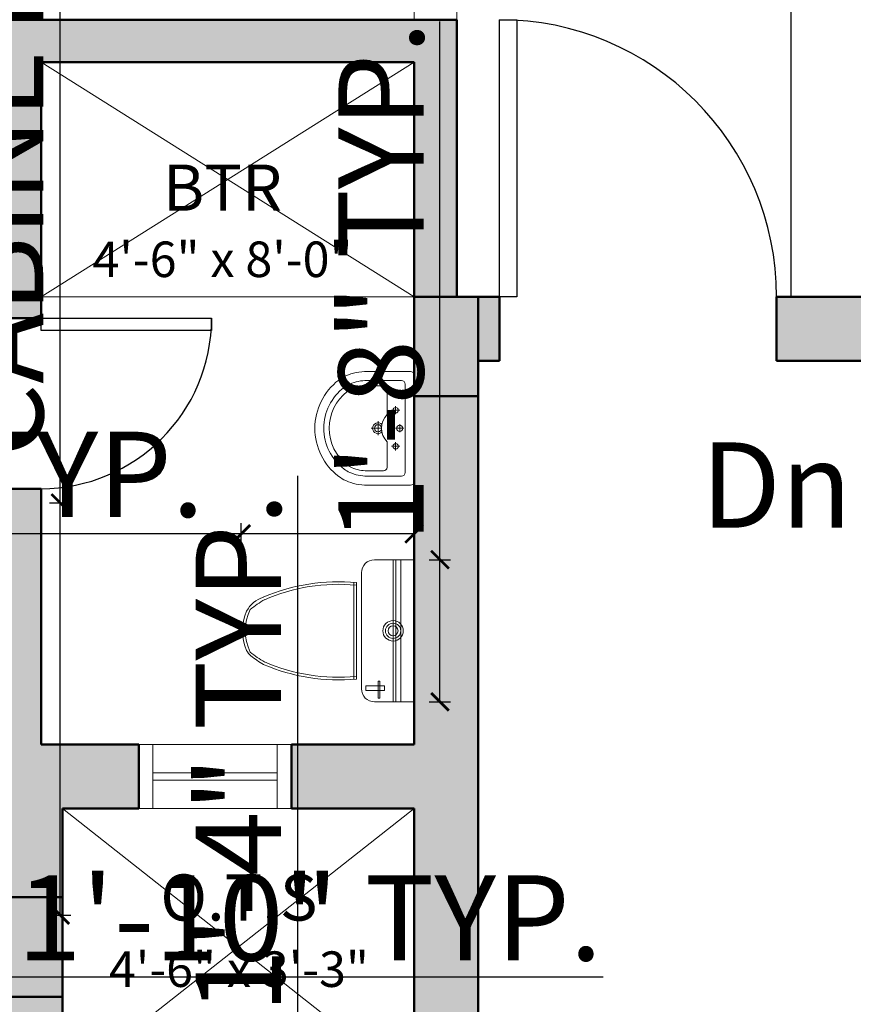
# Model space of a CAD drawing. Units: inches. Extents: x 375 to 1122, y 27 to 1069.
# Tile 80 of 155: x 667 to 784, y 577 to 716. Entities that reach past the tile are written whole.
import ezdxf

# ---------------------------------------------------------------- set-up
doc = ezdxf.new("R2010")
doc.units = ezdxf.units.IN
doc.linetypes.add('ACAD_ISO03W100', pattern=[30, 12, -18])
for name, color, linetype, lineweight in [('A-ANNO-DIMS', 2, 'Continuous', 18), ('A-ANNO-TEXT', 7, 'Continuous', 18), ('A-AREA-IDEN', 7, 'Continuous', 18), ('A-COLS-PATT', 10, 'Continuous', 13), ('A-FLOR-FIXT', 55, 'Continuous', 18), ('A-FLOR-MILL', 55, 'Continuous', 25), ('A-FLOR-OPEN', 250, 'Continuous', 18), ('A-WALL-OVHD', 77, 'ACAD_ISO03W100', 18), ('A-WALL-PATT', 252, 'Continuous', 13), ('Columns', 10, 'Continuous', 50), ('Doors', 150, 'Continuous', 25), ('Shower Areas', 53, 'Continuous', 18), ('Walls', 250, 'Continuous', 50), ('Windows', 122, 'Continuous', 18)]:
    doc.layers.add(name, color=color, linetype=linetype, lineweight=lineweight)
doc.styles.get("Standard").update_dxf_attribs({"font": 'arial.ttf'})
doc.dimstyles.new('ISO-25', dxfattribs={"dimtxt": 12, "dimasz": 2.5, "dimexe": 1.5, "dimexo": 1.5, "dimtad": 1, "dimdec": 1, "dimlunit": 3, "dimtxsty": 'Standard', "dimblk": 'ARCHTICK', "dimcen": 2.5, "dimadec": 0, "dimazin": 0, "dimtfac": 1, "dimtdec": 1, "dimtmove": 0, "dimatfit": 3, "dimfxl": 1.5, "dimfxlon": 1, "dimarcsym": 0})

# ---------------------------------------------------------------- blocks, each defined once
blk = doc.blocks.new('*U4')
for p, q in [((0, 0), (0, -4)), ((28, 0), (28, -4))]:
    blk.add_line(p, q)
blk.add_lwpolyline([(0, 0), (0, 28), (1.75, 28), (1.75, 0)], close=True)
blk.add_arc((0, 0), 28, 0, 90)
blk = doc.blocks.new('*U12')
for p, q in [((0, 0), (0, -4)), ((24, 0), (24, -4))]:
    blk.add_line(p, q)
blk.add_lwpolyline([(0, 0), (0, 24), (1.75, 24), (1.75, 0)], close=True)
blk.add_arc((0, 0), 24, 0, 90)
blk = doc.blocks.new('A$C00C51FE0')
at = {"ltscale": 2}
for p, q in [((16.79, 8.49), (3.21, 8.49)), ((1.85, 7.41), (18.15, 7.41)), ((16.79, 8.12), (3.21, 8.12)), ((0, 0), (0, 5.56)), ((1.59, 4.18), (1.59, 6.81)), ((1.59, 6.81), (2.25, 6.81)), ((2.25, 6.81), (2.25, 4.18)), ((20, 5.56), (20, 0)), ((0.5, 4.84), (0.5, 5.06)), ((0.5, 5.06), (2.91, 5.06)), ((2.91, 4.84), (0.5, 4.84)), ((2.25, 4.18), (1.59, 4.18)), ((2.91, 5.06), (2.91, 4.84)), ((20, 2.96), (0, 2.96)), ((20, 2.59), (0, 2.59)), ((20, 1.85), (0, 1.85)), ((20, 0), (0, 0))]:
    blk.add_line(p, q, dxfattribs=at)
for radius in [1.44, 1.07, 0.698]:
    blk.add_circle((10, 2.96), radius, dxfattribs=at)
for centre, radius, start, end in [((7.96, 21.86), 1.85, 112.9199, 142.816), ((10, 17.03), 6.73, 63.5839, 116.4161), ((10, 17.03), 7.1, 67.0801, 112.9199), ((11.04, 20.15), 3.83, 16.1902, 63.2078), ((22.68, 10.69), 20.34, 142.816, 148.8373), ((22.68, 10.69), 19.97, 141.7352, 148.8373), ((-2.68, 10.69), 19.97, 31.1627, 38.2648), ((29.69, 10.65), 26.6, 156.5869, 185.4494), ((29.69, 10.65), 26.23, 156.5869, 185.4494), ((-9.69, 10.65), 26.23, 354.5506, 23.4131), ((-9.69, 10.65), 26.6, 354.5506, 23.4131), ((1.85, 5.56), 1.85, 90, 180), ((18.15, 5.56), 1.85, 0, 90)]:
    blk.add_arc(centre, radius, start, end, dxfattribs=at)
blk = doc.blocks.new('WINDOW-21_5IN')
for p, q in [((4, 2), (4, 19.5)), ((5, 2), (5, 19.5))]:
    blk.add_line(p, q)
blk.add_lwpolyline([(0, 0), (9, 0), (9, 21.5), (0, 21.5)], close=True)
for points in [[(9, 19.5), (0, 19.5)], [(0, 2), (9, 2)]]:
    blk.add_lwpolyline(points)
blk = doc.blocks.new('LAVATORY-16IN')
for p, q in [((1.78, 12.7), (14.22, 12.7)), ((8, 11.37), (8, 12.51)), ((1.27, 7.37), (1.27, 12.19)), ((4.89, 11.37), (6.03, 11.37)), ((5.46, 10.79), (5.46, 11.94)), ((7.43, 11.94), (8.57, 11.94)), ((9.97, 11.37), (11.11, 11.37)), ((10.54, 10.79), (10.54, 11.94)), ((14.73, 12.19), (14.73, 7.37)), ((2.51, 10.16), (6.08, 10.16)), ((9.91, 10.16), (13.49, 10.16)), ((2.01, 7.37), (2.01, 9.65)), ((7.02, 8.89), (8.98, 8.89)), ((8, 7.91), (8, 9.4)), ((13.99, 9.65), (13.99, 7.37))]:
    blk.add_line(p, q)
blk.add_lwpolyline([(0.51, 13.97), (15.49, 13.97, -0.414214), (16, 13.46), (16, 7.37, -0.104704), (15.37, 4.36, -0.038376), (14.78, 3.36, -0.495903), (1.22, 3.36, -0.038376), (0.63, 4.36, -0.104704), (0, 7.37), (0, 13.46, -0.414214)], format="xyb", close=True)
for points in [[(1.27, 7.37, 0.102694), (1.78, 4.92, 0.037256), (2.25, 4.11, 0.085618)], [(2.01, 7.37, 0.101044), (2.44, 5.24, 0.036381), (2.84, 4.54, 0.084644)], [(13.16, 4.54, 0.036381), (13.56, 5.24, 0.101044), (13.99, 7.37, 0.11083)], [(13.75, 4.11, 0.037256), (14.22, 4.92, 0.102694), (14.73, 7.37, 0.111333)]]:
    blk.add_lwpolyline(points, format="xyb")
for centre, radius in [((5.46, 11.37), 0.381), ((8, 11.94), 0.444), ((10.54, 11.37), 0.381), ((8, 8.89), 0.508)]:
    blk.add_circle(centre, radius)
for centre, radius, start, end in [((1.78, 12.19), 0.508, 90, 180), ((14.22, 12.19), 0.508, 0, 90), ((2.51, 9.65), 0.508, 90, 180), ((7.99, 12.19), 2.79, 226.6581, 313.3419), ((13.49, 9.65), 0.508, 0, 90), ((8, 8.89), 0.762, 133.135, 47.0367), ((8, 8.52), 6.51, 217.6433, 322.3567), ((8, 8.52), 7.25, 217.471, 322.529)]:
    blk.add_arc(centre, radius, start, end)
blk = doc.blocks.new('COLUMN-14X9IN')
blk.add_lwpolyline([(0, 0), (14, 0), (14, 9), (0, 9)], close=True)
blk = doc.blocks.new('SHOWER-PAN-52_5X33IN')
for p, q in [((0, 33), (52.5, 0)), ((52.5, 33), (0, 0))]:
    blk.add_line(p, q)
blk.add_lwpolyline([(0, 0), (52.5, 0), (52.5, 33), (0, 33)], close=True)
blk = doc.blocks.new('_ArchTick')
at = {"color": 0, "linetype": 'ByBlock', "const_width": 0.15}
blk.add_lwpolyline([(-0.5, -0.5), (0.5, 0.5)], dxfattribs=at)
blk = doc.blocks.new('*D45')
at = {"layer": 'A-ANNO-DIMS', "color": 0, "lineweight": -2, "transparency": 16777216}
for p, q in [((697.69, 641.67), (697.69, 644.67)), ((722.01, 641.67), (722.01, 644.67)), ((697.69, 643.17), (559.76, 643.17)), ((722.01, 643.17), (697.69, 643.17))]:
    blk.add_line(p, q, dxfattribs=at)
at = {"layer": 'Defpoints', "color": 0, "transparency": 16777216}
for p in [(697.69, 643.17), (697.69, 639.53), (722.01, 639.53)]:
    blk.add_point(p, dxfattribs=at)
at = {"layer": 'A-ANNO-DIMS', "color": 0, "lineweight": -2, "transparency": 16777216, "xscale": 2.5, "yscale": 2.5, "zscale": 2.5, "rotation": 180}
blk.add_blockref('_ArchTick', (697.69, 643.17), dxfattribs=at)
at = {"layer": 'A-ANNO-DIMS', "color": 0, "lineweight": -2, "transparency": 16777216, "xscale": 2.5, "yscale": 2.5, "zscale": 2.5}
blk.add_blockref('_ArchTick', (722.01, 643.17), dxfattribs=at)
at = {"layer": 'A-ANNO-DIMS', "color": 0, "transparency": 16777216, "insert": (627.47, 650), "char_height": 12, "attachment_point": 5}
blk.add_mtext('WC 2\'-0 1/2" TYP.', dxfattribs=at)
blk = doc.blocks.new('*D46')
at = {"layer": 'A-ANNO-DIMS', "color": 0, "lineweight": -2, "transparency": 16777216}
for p, q in [((725.65, 639.53), (725.65, 715.29)), ((724.15, 639.53), (727.15, 639.53)), ((725.65, 619.53), (725.65, 639.53)), ((724.15, 619.53), (727.15, 619.53))]:
    blk.add_line(p, q, dxfattribs=at)
at = {"layer": 'Defpoints', "color": 0, "transparency": 16777216}
for p in [(722.01, 639.53), (725.65, 639.53), (722.01, 619.53)]:
    blk.add_point(p, dxfattribs=at)
at = {"layer": 'A-ANNO-DIMS', "color": 0, "lineweight": -2, "transparency": 16777216, "xscale": 2.5, "yscale": 2.5, "zscale": 2.5}
for p, rotation in [((725.65, 639.53), 90), ((725.65, 619.53), 270)]:
    blk.add_blockref('_ArchTick', p, dxfattribs=dict(at, rotation=rotation))
at = {"layer": 'A-ANNO-DIMS', "color": 0, "transparency": 16777216, "insert": (718.9, 678.66), "char_height": 12, "attachment_point": 5, "rotation": 90}
blk.add_mtext('1\'-8" TYP.', dxfattribs=at)
blk = doc.blocks.new('*D51')
at = {"layer": 'A-ANNO-DIMS', "color": 0, "lineweight": -2, "transparency": 16777216}
for p, q in [((705.64, 520.03), (705.64, 651.36)), ((706.54, 520.03), (704.14, 520.03)), ((705.64, 504.03), (705.64, 520.03)), ((706.54, 504.03), (704.14, 504.03))]:
    blk.add_line(p, q, dxfattribs=at)
at = {"layer": 'Defpoints', "color": 0, "transparency": 16777216}
for p in [(705.64, 520.03), (708.04, 520.03), (708.04, 504.03)]:
    blk.add_point(p, dxfattribs=at)
at = {"layer": 'A-ANNO-DIMS', "color": 0, "lineweight": -2, "transparency": 16777216, "xscale": 2.5, "yscale": 2.5, "zscale": 2.5}
for p, rotation in [((705.64, 520.03), 90), ((705.64, 504.03), 270)]:
    blk.add_blockref('_ArchTick', p, dxfattribs=dict(at, rotation=rotation))
at = {"layer": 'A-ANNO-DIMS', "color": 0, "transparency": 16777216, "insert": (698.81, 586.94), "char_height": 12, "attachment_point": 5, "rotation": 90}
blk.add_mtext('BASIN 1\'-4" TYP.', dxfattribs=at)
blk = doc.blocks.new('*D57')
at = {"layer": 'A-ANNO-DIMS', "color": 0, "lineweight": -2, "transparency": 16777216}
for p, q in [((512.46, 733.49), (512.46, 730.49)), ((638.07, 733.49), (638.07, 730.49)), ((512.46, 731.99), (638.07, 731.99)), ((638.07, 731.99), (839.76, 731.99))]:
    blk.add_line(p, q, dxfattribs=at)
at = {"layer": 'Defpoints', "color": 0, "transparency": 16777216}
for p in [(512.46, 750.84), (638.07, 750.84), (638.07, 731.99)]:
    blk.add_point(p, dxfattribs=at)
at = {"layer": 'A-ANNO-DIMS', "color": 0, "lineweight": -2, "transparency": 16777216, "xscale": 2.5, "yscale": 2.5, "zscale": 2.5, "rotation": 180}
blk.add_blockref('_ArchTick', (512.46, 731.99), dxfattribs=at)
at = {"layer": 'A-ANNO-DIMS', "color": 0, "lineweight": -2, "transparency": 16777216, "xscale": 2.5, "yscale": 2.5, "zscale": 2.5}
blk.add_blockref('_ArchTick', (638.07, 731.99), dxfattribs=at)
at = {"layer": 'A-ANNO-DIMS', "color": 0, "transparency": 16777216, "insert": (740.16, 738.83), "char_height": 12, "attachment_point": 5}
blk.add_mtext('SOFA SET 10\'-5 1/2" TYP.', dxfattribs=at)
blk = doc.blocks.new('*D79')
at = {"layer": 'A-ANNO-DIMS', "color": 0, "lineweight": -2, "transparency": 16777216}
for p, q in [((672.21, 647.53), (672.21, 810.92)), ((670.71, 647.53), (673.71, 647.53)), ((672.21, 589.53), (672.21, 647.53)), ((670.71, 589.53), (673.71, 589.53))]:
    blk.add_line(p, q, dxfattribs=at)
at = {"layer": 'Defpoints', "color": 0, "transparency": 16777216}
for p in [(663.51, 647.53), (672.21, 647.53), (663.51, 589.53)]:
    blk.add_point(p, dxfattribs=at)
at = {"layer": 'A-ANNO-DIMS', "color": 0, "lineweight": -2, "transparency": 16777216, "xscale": 2.5, "yscale": 2.5, "zscale": 2.5}
for p, rotation in [((672.21, 647.53), 90), ((672.21, 589.53), 270)]:
    blk.add_blockref('_ArchTick', p, dxfattribs=dict(at, rotation=rotation))
at = {"layer": 'A-ANNO-DIMS', "color": 0, "transparency": 16777216, "insert": (665.38, 730.47), "char_height": 12, "attachment_point": 5, "rotation": 90}
blk.add_mtext('CABINET 4\'-10" TYP.', dxfattribs=at)
blk = doc.blocks.new('*D80')
at = {"layer": 'A-ANNO-DIMS', "color": 0, "lineweight": -2, "transparency": 16777216}
for p, q in [((641.51, 582.33), (641.51, 579.33)), ((663.51, 582.33), (663.51, 579.33)), ((641.51, 580.83), (663.51, 580.83)), ((663.51, 580.83), (748.6, 580.83))]:
    blk.add_line(p, q, dxfattribs=at)
at = {"layer": 'Defpoints', "color": 0, "transparency": 16777216}
for p in [(641.51, 589.53), (663.51, 589.53), (663.51, 580.83)]:
    blk.add_point(p, dxfattribs=at)
at = {"layer": 'A-ANNO-DIMS', "color": 0, "lineweight": -2, "transparency": 16777216, "xscale": 2.5, "yscale": 2.5, "zscale": 2.5, "rotation": 180}
blk.add_blockref('_ArchTick', (641.51, 580.83), dxfattribs=at)
at = {"layer": 'A-ANNO-DIMS', "color": 0, "lineweight": -2, "transparency": 16777216, "xscale": 2.5, "yscale": 2.5, "zscale": 2.5}
blk.add_blockref('_ArchTick', (663.51, 580.83), dxfattribs=at)
at = {"layer": 'A-ANNO-DIMS', "color": 0, "transparency": 16777216, "insert": (707.3, 587.58), "char_height": 12, "attachment_point": 5}
blk.add_mtext('1\'-10" TYP.', dxfattribs=at)
blk = doc.blocks.new('*D88')
at = {"layer": 'A-ANNO-DIMS', "color": 0, "lineweight": -2, "transparency": 16777216}
for p, q in [((731.01, 1052.53), (731.01, 1055.53)), ((854.01, 1052.53), (854.01, 1055.53)), ((731.01, 1054.03), (854.01, 1054.03))]:
    blk.add_line(p, q, dxfattribs=at)
at = {"layer": 'Defpoints', "color": 0, "transparency": 16777216}
for p in [(854.01, 1054.03), (731.01, 502.53), (854.01, 502.53)]:
    blk.add_point(p, dxfattribs=at)
at = {"layer": 'A-ANNO-DIMS', "color": 0, "lineweight": -2, "transparency": 16777216, "xscale": 2.5, "yscale": 2.5, "zscale": 2.5, "rotation": 180}
blk.add_blockref('_ArchTick', (731.01, 1054.03), dxfattribs=at)
at = {"layer": 'A-ANNO-DIMS', "color": 0, "lineweight": -2, "transparency": 16777216, "xscale": 2.5, "yscale": 2.5, "zscale": 2.5}
blk.add_blockref('_ArchTick', (854.01, 1054.03), dxfattribs=at)
at = {"layer": 'A-ANNO-DIMS', "color": 0, "transparency": 16777216, "insert": (792.51, 1060.78), "char_height": 12, "attachment_point": 5}
blk.add_mtext('10\'-3"', dxfattribs=at)
blk = doc.blocks.new('*D94')
at = {"layer": 'A-ANNO-DIMS', "color": 0, "lineweight": -2, "transparency": 16777216}
for p, q in [((734.01, 117.53), (734.01, 114.53)), ((773.01, 117.53), (773.01, 114.53)), ((734.01, 116.03), (773.01, 116.03))]:
    blk.add_line(p, q, dxfattribs=at)
at = {"layer": 'Defpoints', "color": 0, "transparency": 16777216}
for p in [(734.01, 667.53), (773.01, 667.53), (773.01, 116.03)]:
    blk.add_point(p, dxfattribs=at)
at = {"layer": 'A-ANNO-DIMS', "color": 0, "lineweight": -2, "transparency": 16777216, "xscale": 2.5, "yscale": 2.5, "zscale": 2.5, "rotation": 180}
blk.add_blockref('_ArchTick', (734.01, 116.03), dxfattribs=at)
at = {"layer": 'A-ANNO-DIMS', "color": 0, "lineweight": -2, "transparency": 16777216, "xscale": 2.5, "yscale": 2.5, "zscale": 2.5}
blk.add_blockref('_ArchTick', (773.01, 116.03), dxfattribs=at)
at = {"layer": 'A-ANNO-DIMS', "color": 0, "transparency": 16777216, "insert": (753.51, 122.78), "char_height": 12, "attachment_point": 5}
blk.add_mtext('3\'-3"', dxfattribs=at)

msp = doc.modelspace()

# ---------------------------------------------------------------- hatches: boundary and pattern name
at = {"layer": 'A-COLS-PATT'}
h = msp.add_hatch(color=256, dxfattribs=at)
h.dxf.hatch_style = 1
h.paths.add_polyline_path([(512.51, 982.53), (498.51, 982.53), (498.51, 973.53), (512.51, 973.53)])
h.paths.add_polyline_path([(666.51, 982.53), (652.51, 982.53), (652.51, 973.53), (666.51, 973.53)])
h.paths.add_polyline_path([(802.01, 982.53), (788.01, 982.53), (788.01, 973.53), (802.01, 973.53)])
h.paths.add_polyline_path([(932.01, 982.53), (918.01, 982.53), (918.01, 973.53), (932.01, 973.53)])
h.paths.add_polyline_path([(507.51, 841.53), (498.51, 841.53), (498.51, 827.53), (507.51, 827.53)])
h.paths.add_polyline_path([(666.51, 844.53), (652.51, 844.53), (652.51, 835.53), (666.51, 835.53)])
h.paths.add_polyline_path([(802.01, 814.53), (788.01, 814.53), (788.01, 805.53), (802.01, 805.53)])
h.paths.add_polyline_path([(932.01, 814.53), (918.01, 814.53), (918.01, 805.53), (932.01, 805.53)])
h.paths.add_polyline_path([(507.51, 719.53), (498.51, 719.53), (498.51, 705.53), (507.51, 705.53)])
h.paths.add_polyline_path([(731.01, 676.53), (722.01, 676.53), (722.01, 662.53), (731.01, 662.53)])
h.paths.add_polyline_path([(802.01, 676.53), (788.01, 676.53), (788.01, 667.53), (802.01, 667.53)])
h.paths.add_polyline_path([(932.01, 676.53), (918.01, 676.53), (918.01, 667.53), (932.01, 667.53)])
h.paths.add_polyline_path([(932.01, 583.53), (918.01, 583.53), (918.01, 574.53), (932.01, 574.53)])
h.paths.add_polyline_path([(868.01, 583.53), (854.01, 583.53), (854.01, 574.53), (868.01, 574.53)])
h.paths.add_polyline_path([(868.01, 502.53), (854.01, 502.53), (854.01, 493.53), (868.01, 493.53)])
h.paths.add_polyline_path([(932.01, 502.53), (918.01, 502.53), (918.01, 493.53), (932.01, 493.53)])
h.paths.add_polyline_path([(672.51, 592.03), (663.51, 592.03), (663.51, 578.03), (672.51, 578.03)])
h.paths.add_polyline_path([(512.51, 589.53), (498.51, 589.53), (498.51, 580.53), (512.51, 580.53)])
h.paths.add_polyline_path([(507.51, 464.53), (498.51, 464.53), (498.51, 450.53), (507.51, 450.53)])
h.paths.add_polyline_path([(731.01, 507.53), (722.01, 507.53), (722.01, 493.53), (731.01, 493.53)])
h.paths.add_polyline_path([(802.01, 502.53), (788.01, 502.53), (788.01, 493.53), (802.01, 493.53)])
h.paths.add_polyline_path([(507.51, 342.53), (498.51, 342.53), (498.51, 328.53), (507.51, 328.53)])
h.paths.add_polyline_path([(512.51, 196.53), (498.51, 196.53), (498.51, 187.53), (512.51, 187.53)])
h.paths.add_polyline_path([(666.51, 334.53), (652.51, 334.53), (652.51, 325.53), (666.51, 325.53)])
h.paths.add_polyline_path([(666.51, 196.53), (652.51, 196.53), (652.51, 187.53), (666.51, 187.53)])
h.paths.add_polyline_path([(805.01, 196.53), (791.01, 196.53), (791.01, 187.53), (805.01, 187.53)])
h.paths.add_polyline_path([(932.01, 196.53), (918.01, 196.53), (918.01, 187.53), (932.01, 187.53)])
h.paths.add_polyline_path([(932.01, 334.53), (918.01, 334.53), (918.01, 325.53), (932.01, 325.53)])
h.paths.add_polyline_path([(805.01, 334.53), (791.01, 334.53), (791.01, 325.53), (805.01, 325.53)])
at = {"layer": 'A-WALL-PATT'}
h = msp.add_hatch(color=256, dxfattribs=at)
h.dxf.hatch_style = 1
h.paths.add_polyline_path([(962.01, 388.53), (989.01, 388.53), (989.01, 394.53), (962.01, 394.53), (932.01, 394.53), (932.01, 397.53), (923.01, 397.53), (923.01, 394.53), (842.01, 394.53), (842.01, 334.53), (839.51, 334.53), (839.51, 328.53), (854.01, 328.53), (854.01, 334.53), (848.01, 334.53), (848.01, 388.53), (953.01, 388.53), (953.01, 356.08), (962.01, 356.08), (962.01, 358.55), (989.01, 358.55), (989.01, 364.55), (962.01, 364.55)])
h.paths.add_polyline_path([(989.01, 502.53), (932.01, 502.53), (932.01, 583.53), (932.01, 593.53), (923.01, 593.53), (923.01, 583.53), (854.01, 583.53), (854.01, 556.53), (863.01, 556.53), (863.01, 574.53), (923.01, 574.53), (923.01, 502.53), (863.01, 502.53), (863.01, 520.53), (854.01, 520.53), (854.01, 502.53), (773.01, 502.53), (773.01, 493.53), (788.01, 493.53), (788.01, 402.03), (722.01, 402.03), (722.01, 373.53), (728.01, 373.53), (728.01, 396.03), (788.01, 396.03), (788.01, 373.53), (794.01, 373.53), (794.01, 430.53), (814.01, 430.53), (814.01, 436.53), (794.01, 436.53), (794.01, 493.53), (923.01, 493.53), (923.01, 487.53), (932.01, 487.53), (932.01, 493.53), (983.01, 493.53), (983.01, 473.53), (989.01, 473.53)])
h.paths.add_polyline_path([(797.01, 325.53), (805.01, 325.53), (805.01, 328.53), (807.51, 328.53), (807.51, 334.53), (791.01, 334.53), (791.01, 226.53), (770.76, 226.53), (770.76, 217.53), (791.01, 217.53), (791.01, 187.53), (855.01, 187.53), (855.01, 196.53), (797.01, 196.53)])
h.paths.add_polyline_path([(989.01, 238.53), (962.01, 238.53), (962.01, 256.42), (953.01, 256.42), (953.01, 229.53), (980.01, 229.53), (980.01, 196.53), (915.01, 196.53), (915.01, 187.53), (989.01, 187.53)])
h.paths.add_polyline_path([(962.01, 334.53), (884.01, 334.53), (884.01, 328.53), (918.01, 328.53), (918.01, 325.53), (932.01, 325.53), (932.01, 328.53), (953.01, 328.53), (953.01, 304.42), (962.01, 304.42)])
h.paths.add_polyline_path([(606.51, 283.53), (609.51, 283.53), (609.51, 289.53), (600.51, 289.53), (600.51, 196.53), (578.51, 196.53), (578.51, 187.53), (606.51, 187.53), (606.51, 196.53)])
h.paths.add_polyline_path([(666.51, 292.53), (660.51, 292.53), (660.51, 289.53), (633.51, 289.53), (633.51, 283.53), (660.51, 283.53), (660.51, 196.53), (628.01, 196.53), (628.01, 187.53), (630.53, 187.53), (630.53, 160.53), (636.53, 160.53), (636.53, 187.53), (660.51, 187.53), (660.51, 160.53), (666.51, 160.53), (666.51, 217.53), (686.76, 217.53), (686.76, 226.53), (666.51, 226.53)])
h.paths.add_polyline_path([(480.51, 256.42), (471.51, 256.42), (471.51, 238.53), (444.51, 238.53), (444.51, 187.53), (518.51, 187.53), (518.51, 196.53), (453.51, 196.53), (453.51, 229.53), (480.51, 229.53)])
h.paths.add_polyline_path([(480.51, 328.53), (652.51, 328.53), (652.51, 325.53), (660.51, 325.53), (660.51, 322.53), (666.51, 322.53), (666.51, 334.53), (507.51, 334.53), (507.51, 360.53), (498.51, 360.53), (498.51, 334.53), (471.51, 334.53), (471.51, 304.42), (480.51, 304.42)])
h.paths.add_polyline_path([(507.51, 484.53), (498.51, 484.53), (498.51, 444.53), (507.51, 444.53), (507.51, 454.53), (621.51, 454.53), (621.51, 460.53), (507.51, 460.53)])
h.paths.add_polyline_path([(672.51, 604.53), (683.26, 604.53), (683.26, 613.53), (669.51, 613.53), (669.51, 649.53), (663.51, 649.53), (663.51, 589.53), (507.51, 589.53), (507.51, 613.53), (498.51, 613.53), (498.51, 556.53), (507.51, 556.53), (507.51, 580.53), (663.51, 580.53), (663.51, 520.53), (669.51, 520.53), (669.51, 556.53), (683.26, 556.53), (683.26, 565.53), (672.51, 565.53)])
h.paths.add_polyline_path([(731.01, 667.53), (734.01, 667.53), (734.01, 676.53), (728.01, 676.53), (728.01, 715.53), (657.51, 715.53), (657.51, 709.53), (663.51, 709.53), (663.51, 673.53), (669.51, 673.53), (669.51, 709.53), (722.01, 709.53), (722.01, 613.53), (704.76, 613.53), (704.76, 604.53), (722.01, 604.53), (722.01, 565.53), (704.76, 565.53), (704.76, 556.53), (722.01, 556.53), (722.01, 502.53), (722.01, 460.53), (669.51, 460.53), (669.51, 496.53), (663.51, 496.53), (663.51, 460.53), (657.51, 460.53), (657.51, 454.53), (728.01, 454.53), (728.01, 493.53), (734.01, 493.53), (734.01, 502.53), (731.01, 502.53)])
h.paths.add_polyline_path([(986.01, 718.53), (959.01, 718.53), (959.01, 727.53), (950.01, 727.53), (950.01, 709.53), (977.01, 709.53), (977.01, 676.53), (794.01, 676.53), (794.01, 805.53), (802.01, 805.53), (802.01, 808.53), (804.51, 808.53), (804.51, 814.53), (788.01, 814.53), (788.01, 774.03), (728.01, 774.03), (728.01, 796.53), (722.01, 796.53), (722.01, 768.03), (788.01, 768.03), (788.01, 676.53), (773.01, 676.53), (773.01, 667.53), (923.01, 667.53), (923.01, 657.53), (932.01, 657.53), (932.01, 667.53), (986.01, 667.53)])
h.paths.add_polyline_path([(621.51, 715.53), (507.51, 715.53), (507.51, 733.53), (498.51, 733.53), (498.51, 715.53), (498.51, 685.53), (507.51, 685.53), (507.51, 709.53), (621.51, 709.53)])
h.paths.add_polyline_path([(666.51, 847.03), (660.51, 847.03), (660.51, 844.53), (652.51, 844.53), (652.51, 841.53), (480.51, 841.53), (480.51, 859.53), (471.51, 859.53), (471.51, 835.53), (498.51, 835.53), (498.51, 817.53), (507.51, 817.53), (507.51, 835.53), (666.51, 835.53)])
h.paths.add_polyline_path([(480.51, 940.53), (453.51, 940.53), (453.51, 973.53), (518.51, 973.53), (518.51, 982.53), (444.51, 982.53), (444.51, 931.53), (471.51, 931.53), (471.51, 907.53), (480.51, 907.53)])
h.paths.add_polyline_path([(606.51, 982.53), (578.51, 982.53), (578.51, 973.53), (600.51, 973.53), (600.51, 880.53), (609.51, 880.53), (609.51, 886.53), (606.51, 886.53)])
h.paths.add_polyline_path([(666.51, 943.53), (686.76, 943.53), (686.76, 952.53), (666.51, 952.53), (666.51, 1009.53), (660.51, 1009.53), (660.51, 982.53), (636.53, 982.53), (636.53, 1009.53), (630.53, 1009.53), (630.53, 982.53), (628.01, 982.53), (628.01, 973.53), (660.51, 973.53), (660.51, 886.53), (633.51, 886.53), (633.51, 880.53), (660.51, 880.53), (660.51, 877.03), (666.51, 877.03)])
h.paths.add_polyline_path([(986.01, 874.53), (932.01, 874.53), (932.01, 877.53), (923.01, 877.53), (923.01, 874.53), (788.01, 874.53), (788.01, 868.53), (788.01, 844.53), (794.01, 844.53), (794.01, 868.53), (839.01, 868.53), (839.01, 814.53), (836.51, 814.53), (836.51, 808.53), (851.01, 808.53), (851.01, 814.53), (845.01, 814.53), (845.01, 868.53), (986.01, 868.53)])
h.paths.add_polyline_path([(959.01, 838.55), (986.01, 838.55), (986.01, 844.55), (959.01, 844.55), (959.01, 847.03), (950.01, 847.03), (950.01, 814.53), (881.01, 814.53), (881.01, 808.53), (918.01, 808.53), (918.01, 805.53), (932.01, 805.53), (932.01, 808.53), (950.01, 808.53), (950.01, 793.53), (959.01, 793.53)])
h.paths.add_polyline_path([(986.01, 982.53), (899.01, 982.53), (899.01, 973.53), (923.01, 973.53), (923.01, 967.53), (932.01, 967.53), (932.01, 973.53), (980.01, 973.53), (980.01, 953.53), (986.01, 953.53)])
h.paths.add_polyline_path([(851.01, 982.53), (788.01, 982.53), (788.01, 952.53), (770.76, 952.53), (770.76, 943.53), (788.01, 943.53), (788.01, 910.53), (814.01, 910.53), (814.01, 916.53), (794.01, 916.53), (794.01, 973.53), (851.01, 973.53)])

# ---------------------------------------------------------------- linework, layer by layer
at = {"layer": 'A-FLOR-MILL'}
msp.add_line((775.01, 768.03), (775.01, 676.53), dxfattribs=at)
at = {"layer": 'A-FLOR-OPEN'}
for p, q in [((672.51, 604.53), (722.01, 565.53)), ((722.01, 604.53), (672.51, 565.53))]:
    msp.add_line(p, q, dxfattribs=at)
at = {"layer": 'A-WALL-OVHD', "ltscale": 0.1}
for p, q in [((722.01, 715.53), (722.01, 768.03)), ((728.01, 715.53), (728.01, 768.03))]:
    msp.add_line(p, q, dxfattribs=at)
at = {"layer": 'Walls'}
for p, q in [((657.51, 715.53), (728.01, 715.53)), ((728.01, 676.53), (728.01, 715.53)), ((669.51, 709.53), (722.01, 709.53)), ((669.51, 673.53), (669.51, 709.53)), ((722.01, 613.53), (722.01, 709.53)), ((734.01, 676.53), (728.01, 676.53)), ((734.01, 676.53), (734.01, 667.53)), ((788.01, 676.53), (773.01, 676.53)), ((773.01, 676.53), (773.01, 667.53)), ((669.51, 673.53), (663.51, 673.53)), ((731.01, 502.53), (731.01, 667.53)), ((734.01, 667.53), (731.01, 667.53)), ((923.01, 667.53), (773.01, 667.53)), ((669.51, 649.53), (663.51, 649.53)), ((669.51, 613.53), (669.51, 649.53)), ((669.51, 613.53), (683.26, 613.53)), ((683.26, 604.53), (683.26, 613.53)), ((704.76, 604.53), (704.76, 613.53)), ((704.76, 613.53), (722.01, 613.53)), ((672.51, 604.53), (683.26, 604.53)), ((672.51, 565.53), (672.51, 604.53)), ((704.76, 604.53), (722.01, 604.53)), ((722.01, 565.53), (722.01, 604.53))]:
    msp.add_line(p, q, dxfattribs=at)

# ---------------------------------------------------------------- block references
at = {"layer": 'A-FLOR-FIXT'}
for name, p, rotation in [('LAVATORY-16IN', (708.04, 666.03), 270), ('A$C00C51FE0', (722.01, 619.53), 89.99999999999999)]:
    msp.add_blockref(name, p, dxfattribs=dict(at, rotation=rotation))
at = {"layer": 'Columns', "rotation": 90}
msp.add_blockref('COLUMN-14X9IN', (731.01, 662.53), dxfattribs=at)
at = {"layer": 'Columns', "extrusion": (0, 0, -1), "zscale": -1, "rotation": 270}
msp.add_blockref('COLUMN-14X9IN', (-672.51, 592.03), dxfattribs=at)
at = {"layer": 'Doors', "xscale": 1.392857142857142, "yscale": 1.392857142857142, "zscale": 1.392857142857142}
msp.add_blockref('*U4', (734.01, 676.53), dxfattribs=at)
at = {"layer": 'Doors', "rotation": 270}
msp.add_blockref('*U12', (669.51, 673.53), dxfattribs=at)
at = {"layer": 'Shower Areas', "extrusion": (0, 0, -1), "zscale": -1, "rotation": 180}
msp.add_blockref('SHOWER-PAN-52_5X33IN', (-669.51, 709.53), dxfattribs=at)
at = {"layer": 'Windows', "rotation": 90}
msp.add_blockref('WINDOW-21_5IN', (704.76, 604.53), dxfattribs=at)

# ---------------------------------------------------------------- texts
at = {"layer": 'A-ANNO-TEXT', "insert": (762.69, 656.04), "char_height": 12, "attachment_point": 1}
msp.add_mtext_dynamic_manual_height_columns('\\pxqc;{\\fArial|b1|i0|c0|p34;Dn}', width=20.5984, gutter_width=12.5, heights=[0], dxfattribs=at)
at = {"layer": 'A-AREA-IDEN', "char_height": 6.5}
for s, insert, attachment_point in [('\\pxqc;{\\fArial|b1|i0|c0|p34;BTR\\P\\fArial|b0|i0|c0|p34;\\H0.76923x;4\'-6" x 8\'-0"}', (673.93, 679.31), 7), ('\\pxqc;{\\fArial|b1|i0|c0|p34;O.T.S\\P\\fArial|b0|i0|c0|p34;\\H0.76923x;4\'-6" x 3\'-3"}', (676.24, 595.25), 1)]:
    msp.add_mtext_dynamic_manual_height_columns(s, width=42.2291, gutter_width=12.5, heights=[0], dxfattribs=dict(at, insert=insert, attachment_point=attachment_point))

# ---------------------------------------------------------------- dimensions: what is measured, and where the dimension line sits
at = {"layer": 'A-ANNO-DIMS'}
for base, p1, p2, picture, middle in [((854.01, 1054.03), (731.01, 502.53), (854.01, 502.53), '*D88', (792.51, 1060.78)), ((773.01, 116.03), (734.01, 667.53), (773.01, 667.53), '*D94', (753.51, 122.78))]:
    dim = msp.add_linear_dim(base=base, p1=p1, p2=p2, dimstyle='ISO-25', override={"dimdec": 1, "dimlfac": 1, "dimrnd": 0, "dimzin": 1, "dimdsep": 46, "dimlunit": 4, "dimfrac": 2}, dxfattribs=at)
    dim.commit()
    dim.dimension.update_dxf_attribs({"geometry": picture, "text_midpoint": middle})
for base, p1, p2, angle, text, picture, middle in [((672.21, 647.53), (663.51, 589.53), (663.51, 647.53), 90, 'CABINET <> TYP.', '*D79', (665.38, 730.47)), ((725.65, 639.53), (722.01, 619.53), (722.01, 639.53), 90, '<> TYP.', '*D46', (718.9, 678.66)), ((697.69, 643.17), (722.01, 639.53), (697.69, 639.53), 180, 'WC <> TYP.', '*D45', (627.47, 650)), ((705.64, 520.03), (708.04, 504.03), (708.04, 520.03), 90, 'BASIN <> TYP.', '*D51', (698.81, 586.94))]:
    dim = msp.add_linear_dim(base=base, p1=p1, p2=p2, angle=angle, text=text, dimstyle='ISO-25', override={"dimdec": 1, "dimlfac": 1, "dimrnd": 0, "dimzin": 1, "dimdsep": 46, "dimlunit": 4, "dimfrac": 2}, dxfattribs=at)
    dim.commit()
    dim.dimension.update_dxf_attribs({"geometry": picture, "text_midpoint": middle})
for base, p1, p2, text, picture, middle in [((638.07, 731.99), (512.46, 750.84), (638.07, 750.84), 'SOFA SET <> TYP.', '*D57', (740.16, 738.83)), ((663.51, 580.83), (641.51, 589.53), (663.51, 589.53), '<> TYP.', '*D80', (707.3, 587.58))]:
    dim = msp.add_linear_dim(base=base, p1=p1, p2=p2, text=text, dimstyle='ISO-25', override={"dimdec": 1, "dimlfac": 1, "dimrnd": 0, "dimzin": 1, "dimdsep": 46, "dimlunit": 4, "dimfrac": 2}, dxfattribs=at)
    dim.commit()
    dim.dimension.update_dxf_attribs({"geometry": picture, "text_midpoint": middle})

doc.saveas('drawing.dxf')
